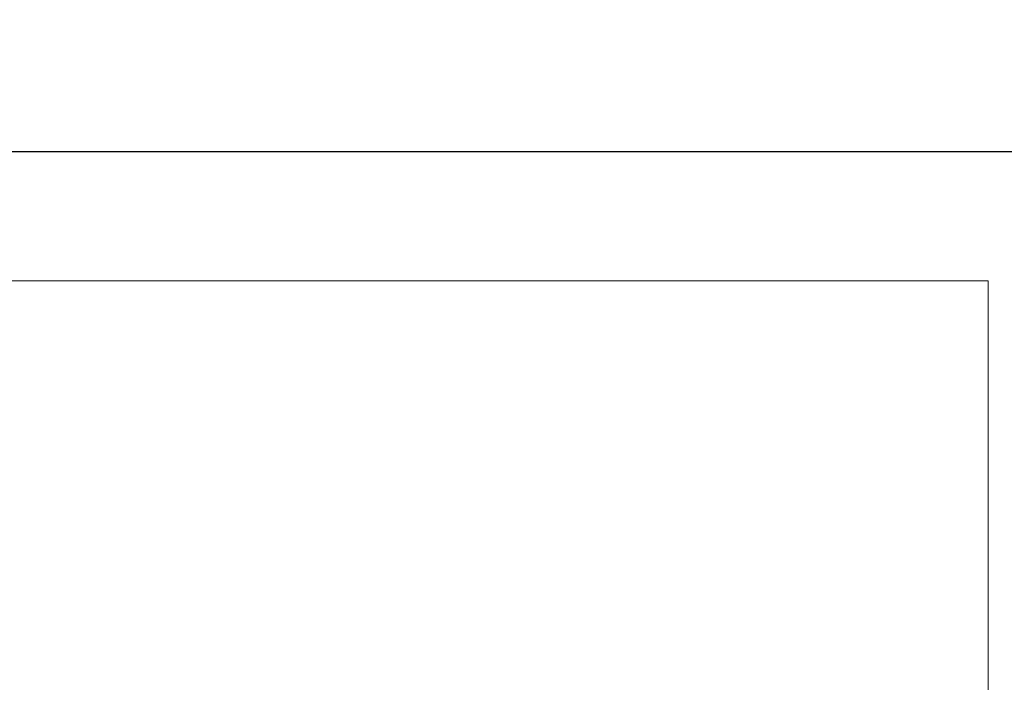
# Model space of a CAD drawing. Units: inches. Extents: x -1198 to -69, y -512 to 437.
# Tile 36 of 50: x -629.007 to -625.117, y 183.132 to 185.749. Entities that reach past the tile are written whole.
import ezdxf

# ---------------------------------------------------------------- set-up
doc = ezdxf.new("R2010")
doc.units = ezdxf.units.IN
doc.header["$MEASUREMENT"] = 0
for name, color, linetype, lineweight in [('0_Pen_No__7', 7, 'Continuous', 18), ('A-ANNO-DIMS', 2, 'Continuous', 18), ('A-EQPM', 60, 'Continuous', 18), ('A-FLOR-CASE', 7, 'Continuous', 25)]:
    doc.layers.add(name, color=color, linetype=linetype, lineweight=lineweight)
doc.styles.get("Standard").update_dxf_attribs({"font": 'arial.ttf'})
doc.dimstyles.get("Standard").update_dxf_attribs({"dimtxt": 6, "dimasz": 6, "dimexe": 0.18, "dimexo": 0.0625, "dimgap": 0.09, "dimtad": 0, "dimtih": 1, "dimtoh": 1, "dimdec": 0, "dimzin": 0, "dimdsep": 46, "dimlunit": 4, "dimtxsty": 'Standard', "dimblk": 'OBLIQUE', "dimcen": 0.09, "dimadec": 0, "dimazin": 0, "dimtfac": 1, "dimtdec": 0, "dimtofl": 0, "dimtmove": 0, "dimatfit": 3, "dimfxl": 1, "dimtolj": 1, "dimtzin": 0, "dimarcsym": 0})

# ---------------------------------------------------------------- blocks, each defined once
blk = doc.blocks.new('new block')
at = {"layer": '0_Pen_No__7'}
blk.add_lwpolyline([(-354.492, 596.906), (481.176, 596.906, -0.414214), (485.681, 592.401), (485.681, 99.109), (486.244, 99.109), (486.244, 95.73), (485.681, 95.73), (485.681, 4.505, -0.414214), (481.176, 0), (-354.492, 0, -0.414214), (-358.997, 4.505), (-358.997, 95.73), (-359.56, 95.73), (-359.56, 99.109), (-358.997, 99.109), (-358.997, 592.401, -0.414214)], format="xyb", close=True, dxfattribs=at)
blk.add_lwpolyline([(-333.701, 12.952), (460.296, 12.952), (460.296, 570.439), (-333.701, 570.439)], close=True, dxfattribs=at)
blk = doc.blocks.new('COUNTER-L')
at = {"ltscale": 10}
blk.add_line((49.3491, 23.9997), (0.0001, 23.9997), dxfattribs=at)
blk = doc.blocks.new('_Oblique')
at = {"color": 0, "linetype": 'ByBlock', "lineweight": -2}
blk.add_line((-0.5, -0.5), (0.5, 0.5), dxfattribs=at)
blk = doc.blocks.new('*D56')
at = {"layer": 'A-ANNO-DIMS', "color": 0, "lineweight": -2, "ltscale": 10, "transparency": 16777216}
for p, q in [((-618.3394, 257.2277), (-603.8219, 257.2277)), ((-604.0019, 257.2277), (-604.0019, 212.422)), ((-604.0019, 161.2277), (-604.0019, 206.0333)), ((-618.3394, 161.2277), (-603.8219, 161.2277))]:
    blk.add_line(p, q, dxfattribs=at)
at = {"layer": 'DEFPOINTS', "color": 0, "ltscale": 10, "transparency": 16777216}
for p in [(-618.4019, 257.2277), (-604.0019, 257.2277), (-618.4019, 161.2277)]:
    blk.add_point(p, dxfattribs=at)
at = {"layer": 'A-ANNO-DIMS', "color": 0, "lineweight": -2, "ltscale": 10, "transparency": 16777216, "xscale": 6, "yscale": 6, "zscale": 6}
for p, rotation in [((-604.0019, 257.2277), 90), ((-604.0019, 161.2277), 270)]:
    blk.add_blockref('_Oblique', p, dxfattribs=dict(at, rotation=rotation))
at = {"layer": 'A-ANNO-DIMS', "color": 0, "ltscale": 10, "transparency": 16777216, "insert": (-604.0019, 209.2277), "char_height": 6, "attachment_point": 5}
blk.add_mtext('\\A1;COUNTER 96 TYP.', dxfattribs=at)

msp = doc.modelspace()

# ---------------------------------------------------------------- block references
at = {"layer": 'A-EQPM', "xscale": 0.0393700787401575, "yscale": 0.0393700787401575, "zscale": 0.0393700787401575, "rotation": 180}
msp.add_blockref('new block', (-638.3186, 185.2277), dxfattribs=at)
at = {"layer": 'A-FLOR-CASE'}
msp.add_blockref('COUNTER-L', (-667.751, 161.228), dxfattribs=at)

# ---------------------------------------------------------------- dimensions: what is measured, and where the dimension line sits
at = {"layer": 'A-ANNO-DIMS', "ltscale": 10}
dim = msp.add_linear_dim(base=(-604.0019, 257.2277), p1=(-618.4019, 161.2277), p2=(-618.4019, 257.2277), angle=90, text='COUNTER <> TYP.', dimstyle='Standard', override={"dimdec": 0, "dimlfac": 1, "dimrnd": 0, "dimzin": 0, "dimdsep": 46, "dimlunit": 2}, dxfattribs=at)
dim.commit()
dim.dimension.update_dxf_attribs({"geometry": '*D56', "text_midpoint": (-604.0019, 209.2277)})

doc.saveas('drawing.dxf')
